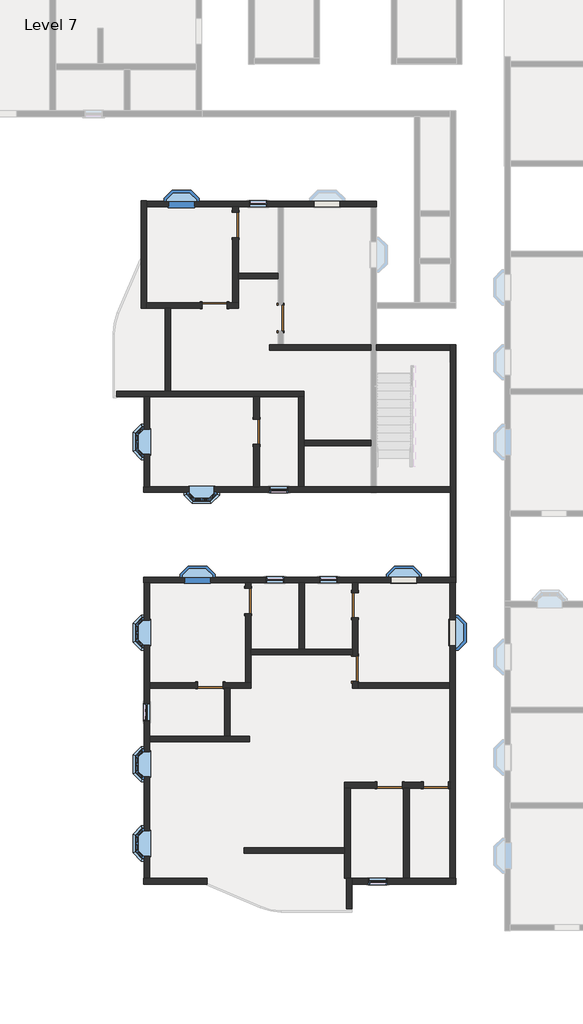
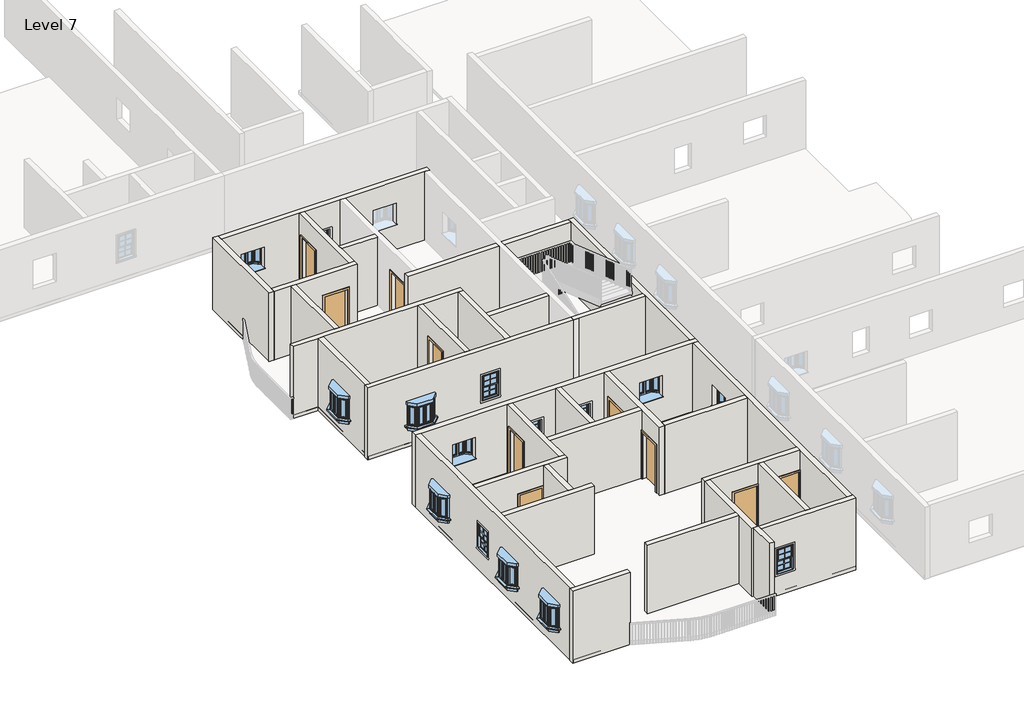
# One storey, part 1 of 14: 32 walls, 15 windows, 10 doors.
"""IFC4 building model written with IfcOpenShell, lengths in millimetres."""

from ifc_helpers import new_model, si_unit, frame, origin, place, context, project, spatial, polyline, outline, extrude, faceted_brep, transform, mapped, element, save
from components import door_54dd4da4, door_719f80de, window_910x910mm_67ef725a, window_8debb0fa

model = new_model("IFC4")

# Units and contexts
model_context = context("Model", 3, world=origin())
ifc_project = project(units=[si_unit("LENGTHUNIT", "METRE", prefix="MILLI")], contexts=[model_context])

# Site, building, storey
site = spatial("IfcSite", under=ifc_project)
building = spatial("IfcBuilding", under=site)
storey = spatial("IfcBuildingStorey", under=building, Name="Level 7", Elevation=18288.0)

# Doors
placement = place(None, origin())
door_shape = door_54dd4da4(model_context)
element("IfcDoor", 1, ObjectType="Single-Flush : 36\" x 84\"", at=placement, inside=storey, context=model_context, shape_type="MappedRepresentation", body=[
    mapped(door_shape, transform((-4626.037215, -17283.4916506, 18288.0), x_axis=(0.0, -1.0, 0.0), y_axis=(1.0, 0.0, 0.0), z_axis=(0.0, 0.0, 1.0))),
])
element("IfcDoor", 2, ObjectType="Single-Flush : 36\" x 84\"", at=placement, inside=storey, context=model_context, shape_type="MappedRepresentation", body=[
    mapped(door_shape, transform((-4626.037215, -14978.4416506, 18288.0), x_axis=(0.0, 1.0, 0.0), y_axis=(-1.0, 0.0, 0.0), z_axis=(0.0, 0.0, 1.0))),
])
element("IfcDoor", 3, ObjectType="Single-Flush : 36\" x 84\"", at=placement, inside=storey, context=model_context, shape_type="MappedRepresentation", body=[
    mapped(door_shape, transform((-9731.437215, -4100.8916506, 18288.0), x_axis=(1.0, 0.0, 0.0), y_axis=(0.0, 1.0, 0.0), z_axis=(0.0, 0.0, 1.0))),
])
element("IfcDoor", 4, ObjectType="Single-Flush : 36\" x 84\"", at=placement, inside=storey, context=model_context, shape_type="MappedRepresentation", body=[
    mapped(door_shape, transform((-7331.137215, -4558.0916506, 18288.0), x_axis=(0.0, -1.0, 0.0), y_axis=(1.0, 0.0, 0.0), z_axis=(0.0, 0.0, 1.0))),
])
door_2_shape = door_719f80de(model_context)
element("IfcDoor", 5, ObjectType="Single-Flush : 36\" x 84\"", at=placement, inside=storey, context=model_context, shape_type="MappedRepresentation", body=[
    mapped(door_2_shape, transform((-9883.837215, -17891.2072331, 18288.0), x_axis=(1.0, 0.0, 0.0), y_axis=(0.0, 1.0, 0.0), z_axis=(0.0, 0.0, 1.0))),
])
element("IfcDoor", 6, ObjectType="Single-Flush : 36\" x 84\"", at=placement, inside=storey, context=model_context, shape_type="MappedRepresentation", body=[
    mapped(door_2_shape, transform((-8512.237215, -14826.0416506, 18288.0), x_axis=(0.0, 1.0, 0.0), y_axis=(-1.0, 0.0, 0.0), z_axis=(0.0, 0.0, 1.0))),
])
element("IfcDoor", 7, ObjectType="Single-Flush : 36\" x 84\"", at=placement, inside=storey, context=model_context, shape_type="MappedRepresentation", body=[
    mapped(door_2_shape, transform((-8207.437215, -8691.9416506, 18288.0), x_axis=(0.0, 1.0, 0.0), y_axis=(-1.0, 0.0, 0.0), z_axis=(0.0, 0.0, 1.0))),
])
element("IfcDoor", 8, ObjectType="Single-Flush : 36\" x 84\"", at=placement, inside=storey, context=model_context, shape_type="MappedRepresentation", body=[
    mapped(door_2_shape, transform((-8969.437215, -1186.2416506, 18288.0), x_axis=(0.0, 1.0, 0.0), y_axis=(-1.0, 0.0, 0.0), z_axis=(0.0, 0.0, 1.0))),
])
element("IfcDoor", 9, ObjectType="Single-Flush : 36\" x 84\"", at=placement, inside=storey, context=model_context, shape_type="MappedRepresentation", body=[
    mapped(door_2_shape, transform((-3374.4891351, -21512.5916506, 18288.0), x_axis=(1.0, 0.0, 0.0), y_axis=(0.0, 1.0, 0.0), z_axis=(0.0, 0.0, 1.0))),
])
element("IfcDoor", 10, ObjectType="Single-Flush : 36\" x 84\"", at=placement, inside=storey, context=model_context, shape_type="MappedRepresentation", body=[
    mapped(door_2_shape, transform((-1698.0891351, -21512.5916506, 18288.0), x_axis=(1.0, 0.0, 0.0), y_axis=(0.0, 1.0, 0.0), z_axis=(0.0, 0.0, 1.0))),
])

# Walls
element("IfcWall", 11, ObjectType="4.5\" p", at=placement, inside=storey, context=model_context, shape_type="Brep", body=[
    faceted_brep([(-9426.637215, -17992.8072331, 20421.6), (-9426.637215, -17992.8072331, 18288.0), (-9375.837215, -17992.8072331, 18288.0), (-9172.637215, -17992.8072331, 18288.0), (-8410.637215, -17992.8072331, 18288.0), (-8410.637215, -17992.8072331, 21336.0), (-9172.637215, -17992.8072331, 21336.0), (-9375.837215, -17992.8072331, 21336.0), (-12087.287215, -17992.8072331, 21336.0), (-12087.287215, -17992.8072331, 18288.0), (-10341.037215, -17992.8072331, 18288.0), (-10341.037215, -17992.8072331, 20421.6), (-8410.637215, -17789.6072331, 18288.0), (-8613.837215, -17789.6072331, 18288.0), (-9426.637215, -17789.6072331, 18288.0), (-9426.637215, -17789.6072331, 20421.6), (-10341.037215, -17789.6072331, 20421.6), (-10341.037215, -17789.6072331, 18288.0), (-12087.287215, -17789.6072331, 18288.0), (-12087.287215, -17789.6072331, 21336.0), (-8613.837215, -17789.6072331, 21336.0), (-8410.637215, -17789.6072331, 21336.0)], [[[0, 1, 2, 3, 4, 5, 6, 7, 8, 9, 10, 11]], [[12, 13, 14, 15, 16, 17, 18, 19, 20, 21]], [[10, 9, 18, 17]], [[4, 3, 2, 1, 14, 13, 12]], [[8, 7, 6, 5, 21, 20, 19]], [[9, 8, 19, 18]], [[5, 4, 12, 21]], [[15, 14, 1, 0]], [[16, 15, 0, 11]], [[17, 16, 11, 10]]]),
])
element("IfcWall", 12, ObjectType="4.5\" p", at=placement, inside=storey, context=model_context, shape_type="Brep", body=[
    faceted_brep([(-8410.637215, -14368.8416506, 20421.6), (-8410.637215, -14368.8416506, 18288.0), (-8410.637215, -14165.6416506, 18288.0), (-8410.637215, -14165.6416506, 21336.0), (-8410.637215, -16572.2916506, 21336.0), (-8410.637215, -16775.4916506, 21336.0), (-8410.637215, -17789.6072331, 21336.0), (-8410.637215, -17789.6072331, 18288.0), (-8410.637215, -16775.4916506, 18288.0), (-8410.637215, -16572.2916506, 18288.0), (-8410.637215, -15283.2416506, 18288.0), (-8410.637215, -15283.2416506, 20421.6), (-8613.837215, -14165.6416506, 18288.0), (-8613.837215, -14368.8416506, 18288.0), (-8613.837215, -14368.8416506, 20421.6), (-8613.837215, -15283.2416506, 20421.6), (-8613.837215, -15283.2416506, 18288.0), (-8613.837215, -17789.6072331, 18288.0), (-8613.837215, -17789.6072331, 21336.0), (-8613.837215, -14165.6416506, 21336.0)], [[[0, 1, 2, 3, 4, 5, 6, 7, 8, 9, 10, 11]], [[12, 13, 14, 15, 16, 17, 18, 19]], [[2, 1, 13, 12]], [[10, 9, 8, 7, 17, 16]], [[6, 5, 4, 3, 19, 18]], [[7, 6, 18, 17]], [[3, 2, 12, 19]], [[14, 13, 1, 0]], [[15, 14, 0, 11]], [[16, 15, 11, 10]]]),
])
element("IfcWall", 13, ObjectType="4.5\" p", at=placement, inside=storey, context=model_context, shape_type="Brep", body=[
    faceted_brep([(-8410.637215, -16775.4916506, 18288.0), (-4727.637215, -16775.4916506, 18288.0), (-4727.637215, -16775.4916506, 21336.0), (-8410.637215, -16775.4916506, 21336.0), (-8410.637215, -16572.2916506, 18288.0), (-8410.637215, -16572.2916506, 21336.0), (-6670.737215, -16572.2916506, 21336.0), (-6467.537215, -16572.2916506, 21336.0), (-4727.637215, -16572.2916506, 21336.0), (-4727.637215, -16572.2916506, 18288.0), (-6467.537215, -16572.2916506, 18288.0), (-6670.737215, -16572.2916506, 18288.0)], [[[0, 1, 2, 3]], [[4, 5, 6, 7, 8, 9, 10, 11]], [[1, 0, 4, 11, 10, 9]], [[3, 2, 8, 7, 6, 5]], [[0, 3, 5, 4]], [[2, 1, 9, 8]]]),
])
element("IfcWall", 14, ObjectType="4.5\" p", at=placement, inside=storey, context=model_context, shape_type="SweptSolid", body=[
    extrude(outline(polyline([(-6670.737215, -16572.2916506), (-6670.737215, -14165.6416506), (-6467.537215, -14165.6416506), (-6467.537215, -16572.2916506), (-6670.737215, -16572.2916506)])), frame((0.0, 0.0, 18288.0), z_axis=(0.0, 0.0, 1.0), x_axis=(1.0, 0.0, 0.0)), (0.0, 0.0, 1.0), 3048.0),
])
element("IfcWall", 15, ObjectType="4.5\" p", at=placement, inside=storey, context=model_context, shape_type="Brep", body=[
    faceted_brep([(-4727.637215, -14165.6416506, 18288.0), (-4727.637215, -14521.2416506, 18288.0), (-4727.637215, -14521.2416506, 20421.6), (-4727.637215, -15435.6416506, 20421.6), (-4727.637215, -15435.6416506, 18288.0), (-4727.637215, -16572.2916506, 18288.0), (-4727.637215, -16775.4916506, 18288.0), (-4727.637215, -16826.2916506, 18288.0), (-4727.637215, -16826.2916506, 20421.6), (-4727.637215, -17740.6916506, 20421.6), (-4727.637215, -17740.6916506, 18288.0), (-4727.637215, -17994.6916506, 18288.0), (-4727.637215, -17994.6916506, 21336.0), (-4727.637215, -16775.4916506, 21336.0), (-4727.637215, -16572.2916506, 21336.0), (-4727.637215, -14165.6416506, 21336.0), (-4524.437215, -14521.2416506, 20421.6), (-4524.437215, -14521.2416506, 18288.0), (-4524.437215, -14165.6416506, 18288.0), (-4524.437215, -14165.6416506, 21336.0), (-4524.437215, -17791.4916506, 21336.0), (-4524.437215, -17994.6916506, 21336.0), (-4524.437215, -17994.6916506, 18288.0), (-4524.437215, -17791.4916506, 18288.0), (-4524.437215, -17740.6916506, 18288.0), (-4524.437215, -17740.6916506, 20421.6), (-4524.437215, -16826.2916506, 20421.6), (-4524.437215, -16826.2916506, 18288.0), (-4524.437215, -15435.6416506, 18288.0), (-4524.437215, -15435.6416506, 20421.6)], [[[0, 1, 2, 3, 4, 5, 6, 7, 8, 9, 10, 11, 12, 13, 14, 15]], [[16, 17, 18, 19, 20, 21, 22, 23, 24, 25, 26, 27, 28, 29]], [[11, 10, 24, 23, 22]], [[28, 27, 7, 6, 5, 4]], [[18, 17, 1, 0]], [[15, 14, 13, 12, 21, 20, 19]], [[0, 15, 19, 18]], [[12, 11, 22, 21]], [[25, 24, 10, 9]], [[26, 25, 9, 8]], [[27, 26, 8, 7]], [[2, 1, 17, 16]], [[3, 2, 16, 29]], [[4, 3, 29, 28]]]),
])
element("IfcWall", 16, ObjectType="4.5\" p", at=placement, inside=storey, context=model_context, shape_type="SweptSolid", body=[
    extrude(outline(polyline([(-4524.437215, -17791.4916506), (-1190.0891351, -17791.4916506), (-1190.0891351, -17994.6916506), (-4524.437215, -17994.6916506), (-4524.437215, -17791.4916506)])), frame((0.0, 0.0, 18288.0), z_axis=(0.0, 0.0, 1.0), x_axis=(1.0, 0.0, 0.0)), (0.0, 0.0, 1.0), 3048.0),
])
element("IfcWall", 17, ObjectType="4.5\" p", at=placement, inside=storey, context=model_context, shape_type="SweptSolid", body=[
    extrude(outline(polyline([(-9375.837215, -19734.5916506), (-9375.837215, -17992.8072331), (-9172.637215, -17992.8072331), (-9172.637215, -19734.5916506), (-9375.837215, -19734.5916506)])), frame((0.0, 0.0, 18288.0), z_axis=(0.0, 0.0, 1.0), x_axis=(1.0, 0.0, 0.0)), (0.0, 0.0, 1.0), 3048.0),
])
element("IfcWall", 18, ObjectType="4.5\" p", at=placement, inside=storey, context=model_context, shape_type="Brep", body=[
    faceted_brep([(-12087.287215, -19937.7916506, 18288.0), (-8455.087215, -19937.7916506, 18288.0), (-8455.087215, -19937.7916506, 21336.0), (-12087.287215, -19937.7916506, 21336.0), (-12087.287215, -19734.5916506, 18288.0), (-12087.287215, -19734.5916506, 21336.0), (-9375.837215, -19734.5916506, 21336.0), (-9172.637215, -19734.5916506, 21336.0), (-8455.087215, -19734.5916506, 21336.0), (-8455.087215, -19734.5916506, 18288.0), (-9172.637215, -19734.5916506, 18288.0), (-9375.837215, -19734.5916506, 18288.0)], [[[0, 1, 2, 3]], [[4, 5, 6, 7, 8, 9, 10, 11]], [[1, 0, 4, 11, 10, 9]], [[2, 1, 9, 8]], [[3, 2, 8, 7, 6, 5]], [[0, 3, 5, 4]]]),
])
element("IfcWall", 19, ObjectType="4.5\" p", at=placement, inside=storey, context=model_context, shape_type="Brep", body=[
    faceted_brep([(-13293.787215, -7421.9416506, 18288.0), (-12290.487215, -7421.9416506, 18288.0), (-12087.287215, -7421.9416506, 18288.0), (-8309.037215, -7421.9416506, 18288.0), (-8105.837215, -7421.9416506, 18288.0), (-6689.787215, -7421.9416506, 18288.0), (-6486.587215, -7421.9416506, 18288.0), (-6486.587215, -7421.9416506, 21336.0), (-6689.787215, -7421.9416506, 21336.0), (-8105.837215, -7421.9416506, 21336.0), (-8309.037215, -7421.9416506, 21336.0), (-12087.287215, -7421.9416506, 21336.0), (-12290.487215, -7421.9416506, 21336.0), (-13293.787215, -7421.9416506, 21336.0), (-13293.787215, -7218.7416506, 18288.0), (-13293.787215, -7218.7416506, 21336.0), (-11528.487215, -7218.7416506, 21336.0), (-11325.287215, -7218.7416506, 21336.0), (-6486.587215, -7218.7416506, 21336.0), (-6486.587215, -7218.7416506, 18288.0), (-11325.287215, -7218.7416506, 18288.0), (-11528.487215, -7218.7416506, 18288.0)], [[[0, 1, 2, 3, 4, 5, 6, 7, 8, 9, 10, 11, 12, 13]], [[14, 15, 16, 17, 18, 19, 20, 21]], [[6, 5, 4, 3, 2, 1, 0, 14, 21, 20, 19]], [[13, 12, 11, 10, 9, 8, 7, 18, 17, 16, 15]], [[0, 13, 15, 14]], [[7, 6, 19, 18]]]),
])
element("IfcWall", 20, ObjectType="4.5\" p", at=placement, inside=storey, context=model_context, shape_type="Brep", body=[
    faceted_brep([(-12201.587215, -4202.4916506, 18288.0), (-12201.587215, -3999.2916506, 18288.0), (-12201.587215, -525.8416506, 18288.0), (-12201.587215, -322.6416506, 18288.0), (-12201.587215, -309.9416506, 18288.0), (-12201.587215, -309.9416506, 21336.0), (-12201.587215, -322.6416506, 21336.0), (-12201.587215, -525.8416506, 21336.0), (-12201.587215, -3999.2916506, 21336.0), (-12201.587215, -4202.4916506, 21336.0), (-12404.787215, -4202.4916506, 18288.0), (-12404.787215, -4202.4916506, 21336.0), (-12404.787215, -309.9416506, 21336.0), (-12404.787215, -309.9416506, 18288.0)], [[[0, 1, 2, 3, 4, 5, 6, 7, 8, 9]], [[10, 11, 12, 13]], [[4, 3, 2, 1, 0, 10, 13]], [[5, 4, 13, 12]], [[9, 8, 7, 6, 5, 12, 11]], [[0, 9, 11, 10]]]),
])
element("IfcWall", 21, ObjectType="4.5\" p", at=placement, inside=storey, context=model_context, shape_type="Brep", body=[
    faceted_brep([(-9274.237215, -4202.4916506, 20421.6), (-9274.237215, -4202.4916506, 18288.0), (-8867.837215, -4202.4916506, 18288.0), (-8867.837215, -4202.4916506, 21336.0), (-11325.287215, -4202.4916506, 21336.0), (-11528.487215, -4202.4916506, 21336.0), (-12201.587215, -4202.4916506, 21336.0), (-12201.587215, -4202.4916506, 18288.0), (-11528.487215, -4202.4916506, 18288.0), (-11325.287215, -4202.4916506, 18288.0), (-10188.637215, -4202.4916506, 18288.0), (-10188.637215, -4202.4916506, 20421.6), (-8867.837215, -3999.2916506, 18288.0), (-9071.037215, -3999.2916506, 18288.0), (-9274.237215, -3999.2916506, 18288.0), (-9274.237215, -3999.2916506, 20421.6), (-10188.637215, -3999.2916506, 20421.6), (-10188.637215, -3999.2916506, 18288.0), (-12201.587215, -3999.2916506, 18288.0), (-12201.587215, -3999.2916506, 21336.0), (-9071.037215, -3999.2916506, 21336.0), (-8867.837215, -3999.2916506, 21336.0)], [[[0, 1, 2, 3, 4, 5, 6, 7, 8, 9, 10, 11]], [[12, 13, 14, 15, 16, 17, 18, 19, 20, 21]], [[2, 1, 14, 13, 12]], [[10, 9, 8, 7, 18, 17]], [[6, 5, 4, 3, 21, 20, 19]], [[7, 6, 19, 18]], [[3, 2, 12, 21]], [[15, 14, 1, 0]], [[16, 15, 0, 11]], [[17, 16, 11, 10]]]),
])
element("IfcWall", 22, ObjectType="4.5\" p", at=placement, inside=storey, context=model_context, shape_type="Brep", body=[
    faceted_brep([(-8867.837215, -729.0416506, 20421.6), (-8867.837215, -729.0416506, 18288.0), (-8867.837215, -525.8416506, 18288.0), (-8867.837215, -525.8416506, 21336.0), (-8867.837215, -2932.4916506, 21336.0), (-8867.837215, -3135.6916506, 21336.0), (-8867.837215, -3999.2916506, 21336.0), (-8867.837215, -3999.2916506, 18288.0), (-8867.837215, -3135.6916506, 18288.0), (-8867.837215, -2932.4916506, 18288.0), (-8867.837215, -1643.4416506, 18288.0), (-8867.837215, -1643.4416506, 20421.6), (-9071.037215, -525.8416506, 18288.0), (-9071.037215, -729.0416506, 18288.0), (-9071.037215, -729.0416506, 20421.6), (-9071.037215, -1643.4416506, 20421.6), (-9071.037215, -1643.4416506, 18288.0), (-9071.037215, -3999.2916506, 18288.0), (-9071.037215, -3999.2916506, 21336.0), (-9071.037215, -525.8416506, 21336.0)], [[[0, 1, 2, 3, 4, 5, 6, 7, 8, 9, 10, 11]], [[12, 13, 14, 15, 16, 17, 18, 19]], [[2, 1, 13, 12]], [[10, 9, 8, 7, 17, 16]], [[6, 5, 4, 3, 19, 18]], [[7, 6, 18, 17]], [[3, 2, 12, 19]], [[14, 13, 1, 0]], [[15, 14, 0, 11]], [[16, 15, 11, 10]]]),
])
element("IfcWall", 23, ObjectType="4.5\" p", at=placement, inside=storey, context=model_context, shape_type="SweptSolid", body=[
    extrude(outline(polyline([(-7432.737215, -3135.6916506), (-8867.837215, -3135.6916506), (-8867.837215, -2932.4916506), (-7432.737215, -2932.4916506), (-7432.737215, -3135.6916506)])), frame((0.0, 0.0, 18288.0), z_axis=(0.0, 0.0, 1.0), x_axis=(1.0, 0.0, 0.0)), (0.0, 0.0, 1.0), 3048.0),
])
element("IfcWall", 24, ObjectType="4.5\" p", at=placement, inside=storey, context=model_context, shape_type="Brep", body=[
    faceted_brep([(-7731.187215, -5726.4916506, 21336.0), (-7731.187215, -5726.4916506, 18288.0), (-4060.887215, -5726.4916506, 18288.0), (-4060.887215, -5726.4916506, 21336.0), (-7731.187215, -5523.2916506, 18288.0), (-7731.187215, -5523.2916506, 21336.0), (-7432.737215, -5523.2916506, 21336.0), (-7229.537215, -5523.2916506, 21336.0), (-4060.887215, -5523.2916506, 21336.0), (-4060.887215, -5523.2916506, 18288.0), (-7229.537215, -5523.2916506, 18288.0), (-7432.737215, -5523.2916506, 18288.0)], [[[0, 1, 2, 3]], [[4, 5, 6, 7, 8, 9, 10, 11]], [[1, 4, 11, 10, 9, 2]], [[5, 0, 3, 8, 7, 6]], [[1, 0, 5, 4]], [[3, 2, 9, 8]]]),
    faceted_brep([(-1177.3891351, -5726.4916506, 18288.0), (-1177.3891351, -5726.4916506, 21336.0), (-3857.687215, -5726.4916506, 21336.0), (-3857.687215, -5726.4916506, 18288.0), (-1177.3891351, -5523.2916506, 21336.0), (-1177.3891351, -5523.2916506, 18288.0), (-3857.687215, -5523.2916506, 18288.0), (-3857.687215, -5523.2916506, 21336.0)], [[[0, 1, 2, 3]], [[4, 5, 6, 7]], [[5, 0, 3, 6]], [[1, 4, 7, 2]], [[1, 0, 5, 4]], [[3, 2, 7, 6]]]),
])
element("IfcWall", 25, ObjectType="4.5\" p", at=placement, inside=storey, context=model_context, shape_type="SweptSolid", body=[
    extrude(outline(polyline([(-11528.487215, -7218.7416506), (-11528.487215, -4202.4916506), (-11325.287215, -4202.4916506), (-11325.287215, -7218.7416506), (-11528.487215, -7218.7416506)])), frame((0.0, 0.0, 18288.0), z_axis=(0.0, 0.0, 1.0), x_axis=(1.0, 0.0, 0.0)), (0.0, 0.0, 1.0), 3048.0),
])
element("IfcWall", 26, ObjectType="4.5\" p", at=placement, inside=storey, context=model_context, shape_type="SweptSolid", body=[
    extrude(outline(polyline([(-7421.9416506, 18288.0), (-8234.7416506, 18288.0), (-8234.7416506, 20421.6), (-9149.1416506, 20421.6), (-9149.1416506, 18288.0), (-10685.8416506, 18288.0), (-10685.8416506, 21336.0), (-7421.9416506, 21336.0), (-7421.9416506, 18288.0)])), frame((-8309.037215, 0.0, 0.0), z_axis=(1.0, 0.0, 0.0), x_axis=(0.0, 1.0, 0.0)), (0.0, 0.0, 1.0), 203.2),
])
element("IfcWall", 27, ObjectType="4.5\" p", at=placement, inside=storey, context=model_context, shape_type="Brep", body=[
    faceted_brep([(-6689.787215, -7421.9416506, 18288.0), (-6689.787215, -10685.8416506, 18288.0), (-6689.787215, -10685.8416506, 21336.0), (-6689.787215, -7421.9416506, 21336.0), (-6486.587215, -7421.9416506, 18288.0), (-6486.587215, -7421.9416506, 21336.0), (-6486.587215, -8990.3916506, 21336.0), (-6486.587215, -9193.5916506, 21336.0), (-6486.587215, -10685.8416506, 21336.0), (-6486.587215, -10685.8416506, 18288.0), (-6486.587215, -9193.5916506, 18288.0), (-6486.587215, -8990.3916506, 18288.0)], [[[0, 1, 2, 3]], [[4, 5, 6, 7, 8, 9, 10, 11]], [[1, 0, 4, 11, 10, 9]], [[3, 2, 8, 7, 6, 5]], [[0, 3, 5, 4]], [[2, 1, 9, 8]]]),
])
element("IfcWall", 28, ObjectType="4.5\" p", at=placement, inside=storey, context=model_context, shape_type="SweptSolid", body=[
    extrude(outline(polyline([(-4060.887215, -9193.5916506), (-6486.587215, -9193.5916506), (-6486.587215, -8990.3916506), (-4060.887215, -8990.3916506), (-4060.887215, -9193.5916506)])), frame((0.0, 0.0, 18288.0), z_axis=(0.0, 0.0, 1.0), x_axis=(1.0, 0.0, 0.0)), (0.0, 0.0, 1.0), 3048.0),
])
element("IfcWall", 29, ObjectType="9\"", at=placement, inside=storey, context=model_context, shape_type="Brep", body=[
    faceted_brep([(-1190.0891351, -21410.9916506, 18288.0), (-1240.8891351, -21410.9916506, 18288.0), (-1240.8891351, -21410.9916506, 20421.6), (-2155.2891351, -21410.9916506, 20421.6), (-2155.2891351, -21410.9916506, 18288.0), (-2917.2891351, -21410.9916506, 18288.0), (-2917.2891351, -21410.9916506, 20421.6), (-3831.6891351, -21410.9916506, 20421.6), (-3831.6891351, -21410.9916506, 18288.0), (-5006.4391351, -21410.9916506, 18288.0), (-5006.4391351, -21410.9916506, 21336.0), (-1190.0891351, -21410.9916506, 21336.0), (-1240.8891351, -21614.1916506, 20421.6), (-1240.8891351, -21614.1916506, 18288.0), (-1190.0891351, -21614.1916506, 18288.0), (-1190.0891351, -21614.1916506, 21336.0), (-2663.2891351, -21614.1916506, 21336.0), (-2866.4891351, -21614.1916506, 21336.0), (-4803.2391351, -21614.1916506, 21336.0), (-5006.4391351, -21614.1916506, 21336.0), (-5006.4391351, -21614.1916506, 18288.0), (-4803.2391351, -21614.1916506, 18288.0), (-3831.6891351, -21614.1916506, 18288.0), (-3831.6891351, -21614.1916506, 20421.6), (-2917.2891351, -21614.1916506, 20421.6), (-2917.2891351, -21614.1916506, 18288.0), (-2866.4891351, -21614.1916506, 18288.0), (-2663.2891351, -21614.1916506, 18288.0), (-2155.2891351, -21614.1916506, 18288.0), (-2155.2891351, -21614.1916506, 20421.6)], [[[0, 1, 2, 3, 4, 5, 6, 7, 8, 9, 10, 11]], [[12, 13, 14, 15, 16, 17, 18, 19, 20, 21, 22, 23, 24, 25, 26, 27, 28, 29]], [[22, 21, 20, 9, 8]], [[14, 13, 1, 0]], [[28, 27, 26, 25, 5, 4]], [[11, 10, 19, 18, 17, 16, 15]], [[0, 11, 15, 14]], [[10, 9, 20, 19]], [[6, 5, 25, 24]], [[7, 6, 24, 23]], [[8, 7, 23, 22]], [[2, 1, 13, 12]], [[3, 2, 12, 29]], [[4, 3, 29, 28]]]),
])
element("IfcWall", 30, ObjectType="9\"", at=placement, inside=storey, context=model_context, shape_type="Brep", body=[
    faceted_brep([(-5006.4391351, -21614.1916506, 18288.0), (-5006.4391351, -23779.5416506, 18288.0), (-5006.4391351, -23982.7416506, 18288.0), (-5006.4391351, -24897.1416506, 18288.0), (-5006.4391351, -24897.1416506, 21336.0), (-5006.4391351, -23982.7416506, 21336.0), (-5006.4391351, -23779.5416506, 21336.0), (-5006.4391351, -21614.1916506, 21336.0), (-4803.2391351, -21614.1916506, 18288.0), (-4803.2391351, -21614.1916506, 21336.0), (-4803.2391351, -24897.1416506, 21336.0), (-4803.2391351, -24897.1416506, 18288.0), (-4949.2891351, -24897.1416506, 18288.0), (-4949.2891351, -24897.1416506, 21336.0)], [[[0, 1, 2, 3, 4, 5, 6, 7]], [[8, 9, 10, 11]], [[3, 2, 1, 0, 8, 11, 12]], [[7, 6, 5, 4, 13, 10, 9]], [[0, 7, 9, 8]], [[4, 3, 12, 11, 10, 13]]]),
])
element("IfcWall", 31, ObjectType="9\"", at=placement, inside=storey, context=model_context, shape_type="SweptSolid", body=[
    extrude(outline(polyline([(-2866.4891351, -24897.1416506), (-2866.4891351, -21614.1916506), (-2663.2891351, -21614.1916506), (-2663.2891351, -24897.1416506), (-2866.4891351, -24897.1416506)])), frame((0.0, 0.0, 18288.0), z_axis=(0.0, 0.0, 1.0), x_axis=(1.0, 0.0, 0.0)), (0.0, 0.0, 1.0), 3048.0),
])
element("IfcWall", 32, ObjectType="9\"", at=placement, inside=storey, context=model_context, shape_type="SweptSolid", body=[
    extrude(outline(polyline([(-5006.4391351, -23982.7416506), (-8664.637215, -23982.7416506), (-8664.637215, -23779.5416506), (-5006.4391351, -23779.5416506), (-5006.4391351, -23982.7416506)])), frame((0.0, 0.0, 18288.0), z_axis=(0.0, 0.0, 1.0), x_axis=(1.0, 0.0, 0.0)), (0.0, 0.0, 1.0), 3048.0),
])
element("IfcWall", 33, ObjectType="9\" w", at=placement, inside=storey, context=model_context, shape_type="Brep", body=[
    faceted_brep([(-12303.187215, -14165.6416506, 18288.0), (-12290.487215, -14165.6416506, 18288.0), (-12087.287215, -14165.6416506, 18288.0), (-8613.837215, -14165.6416506, 18288.0), (-8410.637215, -14165.6416506, 18288.0), (-6670.737215, -14165.6416506, 18288.0), (-6467.537215, -14165.6416506, 18288.0), (-4727.637215, -14165.6416506, 18288.0), (-4524.437215, -14165.6416506, 18288.0), (-1190.0891351, -14165.6416506, 18288.0), (-986.8891351, -14165.6416506, 18288.0), (-961.4891351, -14165.6416506, 18288.0), (-961.4891351, -14165.6416506, 21336.0), (-986.8891351, -14165.6416506, 21336.0), (-1190.0891351, -14165.6416506, 21336.0), (-4524.437215, -14165.6416506, 21336.0), (-4727.637215, -14165.6416506, 21336.0), (-6467.537215, -14165.6416506, 21336.0), (-6670.737215, -14165.6416506, 21336.0), (-8410.637215, -14165.6416506, 21336.0), (-8613.837215, -14165.6416506, 21336.0), (-12087.287215, -14165.6416506, 21336.0), (-12290.487215, -14165.6416506, 21336.0), (-12303.187215, -14165.6416506, 21336.0), (-10805.562215, -14165.6416506, 20398.0), (-9895.562215, -14165.6416506, 20398.0), (-9895.562215, -14165.6416506, 19488.0), (-10805.562215, -14165.6416506, 19488.0), (-3312.2631751, -14165.6416506, 20398.0), (-2402.2631751, -14165.6416506, 20398.0), (-2402.2631751, -14165.6416506, 19488.0), (-3312.2631751, -14165.6416506, 19488.0), (-7870.887215, -14165.6416506, 20269.2), (-7210.487215, -14165.6416506, 20269.2), (-7210.487215, -14165.6416506, 19202.4), (-7870.887215, -14165.6416506, 19202.4), (-5927.787215, -14165.6416506, 20269.2), (-5267.387215, -14165.6416506, 20269.2), (-5267.387215, -14165.6416506, 19202.4), (-5927.787215, -14165.6416506, 19202.4), (-12303.187215, -13962.4416506, 18288.0), (-12303.187215, -13962.4416506, 21336.0), (-1177.3891351, -13962.4416506, 21336.0), (-974.1891351, -13962.4416506, 21336.0), (-961.4891351, -13962.4416506, 21336.0), (-961.4891351, -13962.4416506, 18288.0), (-974.1891351, -13962.4416506, 18288.0), (-1177.3891351, -13962.4416506, 18288.0), (-10805.562215, -13962.4416506, 20398.0), (-10805.562215, -13962.4416506, 19488.0), (-9895.562215, -13962.4416506, 19488.0), (-9895.562215, -13962.4416506, 20398.0), (-3312.2631751, -13962.4416506, 20398.0), (-3312.2631751, -13962.4416506, 19488.0), (-2402.2631751, -13962.4416506, 19488.0), (-2402.2631751, -13962.4416506, 20398.0), (-7870.887215, -13962.4416506, 20269.2), (-7870.887215, -13962.4416506, 19202.4), (-7210.487215, -13962.4416506, 19202.4), (-7210.487215, -13962.4416506, 20269.2), (-5927.787215, -13962.4416506, 20269.2), (-5927.787215, -13962.4416506, 19202.4), (-5267.387215, -13962.4416506, 19202.4), (-5267.387215, -13962.4416506, 20269.2)], [[[0, 1, 2, 3, 4, 5, 6, 7, 8, 9, 10, 11, 12, 13, 14, 15, 16, 17, 18, 19, 20, 21, 22, 23], [24, 25, 26, 27], [28, 29, 30, 31], [32, 33, 34, 35], [36, 37, 38, 39]], [[40, 41, 42, 43, 44, 45, 46, 47], [48, 49, 50, 51], [52, 53, 54, 55], [56, 57, 58, 59], [60, 61, 62, 63]], [[11, 10, 9, 8, 7, 6, 5, 4, 3, 2, 1, 0, 40, 47, 46, 45]], [[12, 11, 45, 44]], [[23, 22, 21, 20, 19, 18, 17, 16, 15, 14, 13, 12, 44, 43, 42, 41]], [[0, 23, 41, 40]], [[49, 48, 24, 27]], [[50, 49, 27, 26]], [[51, 50, 26, 25]], [[48, 51, 25, 24]], [[53, 52, 28, 31]], [[54, 53, 31, 30]], [[55, 54, 30, 29]], [[52, 55, 29, 28]], [[57, 56, 32, 35]], [[58, 57, 35, 34]], [[59, 58, 34, 33]], [[56, 59, 33, 32]], [[61, 60, 36, 39]], [[62, 61, 39, 38]], [[63, 62, 38, 37]], [[60, 63, 37, 36]]]),
])
element("IfcWall", 34, ObjectType="9\" w", at=placement, inside=storey, context=model_context, shape_type="Brep", body=[
    faceted_brep([(-10004.0323936, -24897.1416506, 18288.0), (-12087.287215, -24897.1416506, 18288.0), (-12290.487215, -24897.1416506, 18288.0), (-12303.187215, -24897.1416506, 18288.0), (-12303.187215, -24897.1416506, 21336.0), (-12290.487215, -24897.1416506, 21336.0), (-12087.287215, -24897.1416506, 21336.0), (-10004.0323936, -24897.1416506, 21336.0), (-10004.0323936, -25100.3416506, 18288.0), (-10004.0323936, -25100.3416506, 21336.0), (-12303.187215, -25100.3416506, 21336.0), (-12303.187215, -25100.3416506, 18288.0)], [[[0, 1, 2, 3, 4, 5, 6, 7]], [[8, 9, 10, 11]], [[3, 2, 1, 0, 8, 11]], [[4, 3, 11, 10]], [[7, 6, 5, 4, 10, 9]], [[0, 7, 9, 8]]]),
])
element("IfcWall", 35, ObjectType="9\" w", at=placement, inside=storey, context=model_context, shape_type="Brep", body=[
    faceted_brep([(-4746.0891351, -25989.3416506, 18288.0), (-4746.0891351, -25100.3416506, 18288.0), (-4746.0891351, -24897.1416506, 18288.0), (-4746.0891351, -24897.1416506, 21336.0), (-4746.0891351, -25100.3416506, 21336.0), (-4746.0891351, -25989.3416506, 21336.0), (-4949.2891351, -25989.3416506, 18288.0), (-4949.2891351, -25989.3416506, 21336.0), (-4949.2891351, -24897.1416506, 21336.0), (-4949.2891351, -24897.1416506, 18288.0), (-4803.2391351, -24897.1416506, 18288.0), (-4803.2391351, -24897.1416506, 21336.0)], [[[0, 1, 2, 3, 4, 5]], [[6, 7, 8, 9]], [[2, 1, 0, 6, 9, 10]], [[5, 4, 3, 11, 8, 7]], [[0, 5, 7, 6]], [[3, 2, 10, 9, 8, 11]]]),
])
element("IfcWall", 36, ObjectType="9\" w", at=placement, inside=storey, context=model_context, shape_type="Brep", body=[
    faceted_brep([(-4746.0891351, -25100.3416506, 18288.0), (-961.4891351, -25100.3416506, 18288.0), (-961.4891351, -25100.3416506, 21336.0), (-4746.0891351, -25100.3416506, 21336.0), (-3476.0891351, -25100.3416506, 20269.2), (-3476.0891351, -25100.3416506, 19202.4), (-4136.4891351, -25100.3416506, 19202.4), (-4136.4891351, -25100.3416506, 20269.2), (-4746.0891351, -24897.1416506, 18288.0), (-4746.0891351, -24897.1416506, 21336.0), (-2866.4891351, -24897.1416506, 21336.0), (-2663.2891351, -24897.1416506, 21336.0), (-1190.0891351, -24897.1416506, 21336.0), (-986.8891351, -24897.1416506, 21336.0), (-961.4891351, -24897.1416506, 21336.0), (-961.4891351, -24897.1416506, 18288.0), (-986.8891351, -24897.1416506, 18288.0), (-1190.0891351, -24897.1416506, 18288.0), (-2663.2891351, -24897.1416506, 18288.0), (-2866.4891351, -24897.1416506, 18288.0), (-3476.0891351, -24897.1416506, 20269.2), (-4136.4891351, -24897.1416506, 20269.2), (-4136.4891351, -24897.1416506, 19202.4), (-3476.0891351, -24897.1416506, 19202.4)], [[[0, 1, 2, 3], [4, 5, 6, 7]], [[8, 9, 10, 11, 12, 13, 14, 15, 16, 17, 18, 19], [20, 21, 22, 23]], [[1, 0, 8, 19, 18, 17, 16, 15]], [[2, 1, 15, 14]], [[3, 2, 14, 13, 12, 11, 10, 9]], [[0, 3, 9, 8]], [[5, 4, 20, 23]], [[6, 5, 23, 22]], [[7, 6, 22, 21]], [[4, 7, 21, 20]]]),
])
element("IfcWall", 37, ObjectType="9\" w", at=placement, inside=storey, context=model_context, shape_type="Brep", body=[
    faceted_brep([(-12290.487215, -14165.6416506, 18288.0), (-12290.487215, -24897.1416506, 18288.0), (-12290.487215, -24897.1416506, 21336.0), (-12290.487215, -14165.6416506, 21336.0), (-12290.487215, -16432.6244419, 20112.4), (-12290.487215, -16432.6244419, 19202.4), (-12290.487215, -15522.6244419, 19202.4), (-12290.487215, -15522.6244419, 20112.4), (-12290.487215, -21205.5916506, 20112.4), (-12290.487215, -21205.5916506, 19202.4), (-12290.487215, -20295.5916506, 19202.4), (-12290.487215, -20295.5916506, 20112.4), (-12290.487215, -24082.1416506, 20112.4), (-12290.487215, -24082.1416506, 19202.4), (-12290.487215, -23172.1416506, 19202.4), (-12290.487215, -23172.1416506, 20112.4), (-12290.487215, -19193.8994419, 20269.2), (-12290.487215, -19193.8994419, 19202.4), (-12290.487215, -18533.4994419, 19202.4), (-12290.487215, -18533.4994419, 20269.2), (-12087.287215, -14165.6416506, 18288.0), (-12087.287215, -14165.6416506, 21336.0), (-12087.287215, -17789.6072331, 21336.0), (-12087.287215, -17992.8072331, 21336.0), (-12087.287215, -19734.5916506, 21336.0), (-12087.287215, -19937.7916506, 21336.0), (-12087.287215, -24897.1416506, 21336.0), (-12087.287215, -24897.1416506, 18288.0), (-12087.287215, -19937.7916506, 18288.0), (-12087.287215, -19734.5916506, 18288.0), (-12087.287215, -17992.8072331, 18288.0), (-12087.287215, -17789.6072331, 18288.0), (-12087.287215, -16432.6244419, 20112.4), (-12087.287215, -15522.6244419, 20112.4), (-12087.287215, -15522.6244419, 19202.4), (-12087.287215, -16432.6244419, 19202.4), (-12087.287215, -21205.5916506, 20112.4), (-12087.287215, -20295.5916506, 20112.4), (-12087.287215, -20295.5916506, 19202.4), (-12087.287215, -21205.5916506, 19202.4), (-12087.287215, -24082.1416506, 20112.4), (-12087.287215, -23172.1416506, 20112.4), (-12087.287215, -23172.1416506, 19202.4), (-12087.287215, -24082.1416506, 19202.4), (-12087.287215, -19193.8994419, 20269.2), (-12087.287215, -18533.4994419, 20269.2), (-12087.287215, -18533.4994419, 19202.4), (-12087.287215, -19193.8994419, 19202.4)], [[[0, 1, 2, 3], [4, 5, 6, 7], [8, 9, 10, 11], [12, 13, 14, 15], [16, 17, 18, 19]], [[20, 21, 22, 23, 24, 25, 26, 27, 28, 29, 30, 31], [32, 33, 34, 35], [36, 37, 38, 39], [40, 41, 42, 43], [44, 45, 46, 47]], [[1, 0, 20, 31, 30, 29, 28, 27]], [[3, 2, 26, 25, 24, 23, 22, 21]], [[0, 3, 21, 20]], [[2, 1, 27, 26]], [[5, 4, 32, 35]], [[6, 5, 35, 34]], [[7, 6, 34, 33]], [[4, 7, 33, 32]], [[9, 8, 36, 39]], [[10, 9, 39, 38]], [[11, 10, 38, 37]], [[8, 11, 37, 36]], [[13, 12, 40, 43]], [[14, 13, 43, 42]], [[15, 14, 42, 41]], [[12, 15, 41, 40]], [[17, 16, 44, 47]], [[18, 17, 47, 46]], [[19, 18, 46, 45]], [[16, 19, 45, 44]]]),
])
element("IfcWall", 38, ObjectType="9\" w", at=placement, inside=storey, context=model_context, shape_type="Brep", body=[
    faceted_brep([(-1190.0891351, -14165.6416506, 18288.0), (-1190.0891351, -17791.4916506, 18288.0), (-1190.0891351, -17994.6916506, 18288.0), (-1190.0891351, -21410.9916506, 18288.0), (-1190.0891351, -21614.1916506, 18288.0), (-1190.0891351, -24897.1416506, 18288.0), (-1190.0891351, -24897.1416506, 21336.0), (-1190.0891351, -21614.1916506, 21336.0), (-1190.0891351, -21410.9916506, 21336.0), (-1190.0891351, -17994.6916506, 21336.0), (-1190.0891351, -17791.4916506, 21336.0), (-1190.0891351, -14165.6416506, 21336.0), (-1190.0891351, -15523.5666506, 20398.0), (-1190.0891351, -16433.5666506, 20398.0), (-1190.0891351, -16433.5666506, 19488.0), (-1190.0891351, -15523.5666506, 19488.0), (-986.8891351, -14165.6416506, 18288.0), (-986.8891351, -14165.6416506, 21336.0), (-986.8891351, -24897.1416506, 21336.0), (-986.8891351, -24897.1416506, 18288.0), (-986.8891351, -15523.5666506, 20398.0), (-986.8891351, -15523.5666506, 19488.0), (-986.8891351, -16433.5666506, 19488.0), (-986.8891351, -16433.5666506, 20398.0)], [[[0, 1, 2, 3, 4, 5, 6, 7, 8, 9, 10, 11], [12, 13, 14, 15]], [[16, 17, 18, 19], [20, 21, 22, 23]], [[5, 4, 3, 2, 1, 0, 16, 19]], [[11, 10, 9, 8, 7, 6, 18, 17]], [[0, 11, 17, 16]], [[6, 5, 19, 18]], [[21, 20, 12, 15]], [[22, 21, 15, 14]], [[23, 22, 14, 13]], [[20, 23, 13, 12]]]),
])
element("IfcWall", 39, ObjectType="9\" w", at=placement, inside=storey, context=model_context, shape_type="Brep", body=[
    faceted_brep([(-1177.3891351, -5523.2916506, 18288.0), (-1177.3891351, -5726.4916506, 18288.0), (-1177.3891351, -10685.8416506, 18288.0), (-1177.3891351, -10889.0416506, 18288.0), (-1177.3891351, -13962.4416506, 18288.0), (-1177.3891351, -13962.4416506, 21336.0), (-1177.3891351, -10889.0416506, 21336.0), (-1177.3891351, -10685.8416506, 21336.0), (-1177.3891351, -5726.4916506, 21336.0), (-1177.3891351, -5523.2916506, 21336.0), (-974.1891351, -5523.2916506, 18288.0), (-974.1891351, -5523.2916506, 21336.0), (-974.1891351, -13962.4416506, 21336.0), (-974.1891351, -13962.4416506, 18288.0)], [[[0, 1, 2, 3, 4, 5, 6, 7, 8, 9]], [[10, 11, 12, 13]], [[4, 3, 2, 1, 0, 10, 13]], [[9, 8, 7, 6, 5, 12, 11]], [[5, 4, 13, 12]], [[0, 9, 11, 10]]]),
])
element("IfcWall", 40, ObjectType="9\" w", at=placement, inside=storey, context=model_context, shape_type="Brep", body=[
    faceted_brep([(-1177.3891351, -10685.8416506, 18288.0), (-6486.587215, -10685.8416506, 18288.0), (-6689.787215, -10685.8416506, 18288.0), (-8105.837215, -10685.8416506, 18288.0), (-8309.037215, -10685.8416506, 18288.0), (-12087.287215, -10685.8416506, 18288.0), (-12290.487215, -10685.8416506, 18288.0), (-12303.187215, -10685.8416506, 18288.0), (-12303.187215, -10685.8416506, 21336.0), (-12290.487215, -10685.8416506, 21336.0), (-12087.287215, -10685.8416506, 21336.0), (-8309.037215, -10685.8416506, 21336.0), (-8105.837215, -10685.8416506, 21336.0), (-6689.787215, -10685.8416506, 21336.0), (-6486.587215, -10685.8416506, 21336.0), (-1177.3891351, -10685.8416506, 21336.0), (-9743.162215, -10685.8416506, 20112.4), (-10653.162215, -10685.8416506, 20112.4), (-10653.162215, -10685.8416506, 19202.4), (-9743.162215, -10685.8416506, 19202.4), (-7067.612215, -10685.8416506, 20269.2), (-7728.012215, -10685.8416506, 20269.2), (-7728.012215, -10685.8416506, 19202.4), (-7067.612215, -10685.8416506, 19202.4), (-1177.3891351, -10889.0416506, 18288.0), (-1177.3891351, -10889.0416506, 21336.0), (-12303.187215, -10889.0416506, 21336.0), (-12303.187215, -10889.0416506, 18288.0), (-9743.162215, -10889.0416506, 20112.4), (-9743.162215, -10889.0416506, 19202.4), (-10653.162215, -10889.0416506, 19202.4), (-10653.162215, -10889.0416506, 20112.4), (-7067.612215, -10889.0416506, 20269.2), (-7067.612215, -10889.0416506, 19202.4), (-7728.012215, -10889.0416506, 19202.4), (-7728.012215, -10889.0416506, 20269.2)], [[[0, 1, 2, 3, 4, 5, 6, 7, 8, 9, 10, 11, 12, 13, 14, 15], [16, 17, 18, 19], [20, 21, 22, 23]], [[24, 25, 26, 27], [28, 29, 30, 31], [32, 33, 34, 35]], [[7, 6, 5, 4, 3, 2, 1, 0, 24, 27]], [[8, 7, 27, 26]], [[15, 14, 13, 12, 11, 10, 9, 8, 26, 25]], [[0, 15, 25, 24]], [[29, 28, 16, 19]], [[30, 29, 19, 18]], [[31, 30, 18, 17]], [[28, 31, 17, 16]], [[33, 32, 20, 23]], [[34, 33, 23, 22]], [[35, 34, 22, 21]], [[32, 35, 21, 20]]]),
])
element("IfcWall", 41, ObjectType="9\" w", at=placement, inside=storey, context=model_context, shape_type="SweptSolid", body=[
    extrude(outline(polyline([(-10685.8416506, 18288.0), (-10685.8416506, 21336.0), (-7421.9416506, 21336.0), (-7421.9416506, 18288.0), (-10685.8416506, 18288.0)]), holes=[polyline([(-9508.8916506, 20112.4), (-9508.8916506, 19202.4), (-8598.8916506, 19202.4), (-8598.8916506, 20112.4), (-9508.8916506, 20112.4)])]), frame((-12290.487215, 0.0, 0.0), z_axis=(1.0, 0.0, 0.0), x_axis=(0.0, 1.0, 0.0)), (0.0, 0.0, 1.0), 203.2),
])
element("IfcWall", 42, ObjectType="9\" w", at=placement, inside=storey, context=model_context, shape_type="Brep", body=[
    faceted_brep([(-12201.587215, -525.8416506, 18288.0), (-9071.037215, -525.8416506, 18288.0), (-8867.837215, -525.8416506, 18288.0), (-7432.737215, -525.8416506, 18288.0), (-7229.537215, -525.8416506, 18288.0), (-4060.887215, -525.8416506, 18288.0), (-3857.687215, -525.8416506, 18288.0), (-3844.987215, -525.8416506, 18288.0), (-3844.987215, -525.8416506, 21336.0), (-3857.687215, -525.8416506, 21336.0), (-4060.887215, -525.8416506, 21336.0), (-7229.537215, -525.8416506, 21336.0), (-7432.737215, -525.8416506, 21336.0), (-8867.837215, -525.8416506, 21336.0), (-9071.037215, -525.8416506, 21336.0), (-12201.587215, -525.8416506, 21336.0), (-6100.212215, -525.8416506, 20398.0), (-5190.212215, -525.8416506, 20398.0), (-5190.212215, -525.8416506, 19488.0), (-6100.212215, -525.8416506, 19488.0), (-11386.587215, -525.8416506, 20398.0), (-10476.587215, -525.8416506, 20398.0), (-10476.587215, -525.8416506, 19488.0), (-11386.587215, -525.8416506, 19488.0), (-8480.487215, -525.8416506, 20269.2), (-7820.087215, -525.8416506, 20269.2), (-7820.087215, -525.8416506, 19202.4), (-8480.487215, -525.8416506, 19202.4), (-12201.587215, -322.6416506, 18288.0), (-12201.587215, -322.6416506, 21336.0), (-3844.987215, -322.6416506, 21336.0), (-3844.987215, -322.6416506, 18288.0), (-6100.212215, -322.6416506, 20398.0), (-6100.212215, -322.6416506, 19488.0), (-5190.212215, -322.6416506, 19488.0), (-5190.212215, -322.6416506, 20398.0), (-11386.587215, -322.6416506, 20398.0), (-11386.587215, -322.6416506, 19488.0), (-10476.587215, -322.6416506, 19488.0), (-10476.587215, -322.6416506, 20398.0), (-8480.487215, -322.6416506, 20269.2), (-8480.487215, -322.6416506, 19202.4), (-7820.087215, -322.6416506, 19202.4), (-7820.087215, -322.6416506, 20269.2)], [[[0, 1, 2, 3, 4, 5, 6, 7, 8, 9, 10, 11, 12, 13, 14, 15], [16, 17, 18, 19], [20, 21, 22, 23], [24, 25, 26, 27]], [[28, 29, 30, 31], [32, 33, 34, 35], [36, 37, 38, 39], [40, 41, 42, 43]], [[7, 6, 5, 4, 3, 2, 1, 0, 28, 31]], [[8, 7, 31, 30]], [[15, 14, 13, 12, 11, 10, 9, 8, 30, 29]], [[0, 15, 29, 28]], [[33, 32, 16, 19]], [[34, 33, 19, 18]], [[35, 34, 18, 17]], [[32, 35, 17, 16]], [[37, 36, 20, 23]], [[38, 37, 23, 22]], [[39, 38, 22, 21]], [[36, 39, 21, 20]], [[41, 40, 24, 27]], [[42, 41, 27, 26]], [[43, 42, 26, 25]], [[40, 43, 25, 24]]]),
])

# Windows
window_910x910mm_shape = window_910x910mm_67ef725a(model_context)
element("IfcWindow", 43, ObjectType="910x910mm", at=placement, inside=storey, context=model_context, shape_type="MappedRepresentation", body=[
    mapped(window_910x910mm_shape, transform((-10361.587215, -432.6982184, 18288.0), x_axis=(1.0, 0.0, 0.0), y_axis=(0.0, 1.0, 0.0), z_axis=(0.0, 0.0, 1.0))),
])
element("IfcWindow", 44, ObjectType="910x910mm", at=placement, inside=storey, context=model_context, shape_type="MappedRepresentation", body=[
    mapped(window_910x910mm_shape, transform((-12180.4306471, -8483.8916506, 18002.4), x_axis=(0.0, 1.0, 0.0), y_axis=(-1.0, 0.0, 0.0), z_axis=(0.0, 0.0, 1.0))),
])
element("IfcWindow", 45, ObjectType="910x910mm", at=placement, inside=storey, context=model_context, shape_type="MappedRepresentation", body=[
    mapped(window_910x910mm_shape, transform((-10768.162215, -10778.9850828, 18002.4), x_axis=(-1.0, 0.0, 0.0), y_axis=(0.0, -1.0, 0.0), z_axis=(0.0, 0.0, 1.0))),
])
element("IfcWindow", 46, ObjectType="910x910mm", at=placement, inside=storey, context=model_context, shape_type="MappedRepresentation", body=[
    mapped(window_910x910mm_shape, transform((-12180.4306471, -15407.6244419, 18002.4), x_axis=(0.0, 1.0, 0.0), y_axis=(-1.0, 0.0, 0.0), z_axis=(0.0, 0.0, 1.0))),
])
element("IfcWindow", 47, ObjectType="910x910mm", at=placement, inside=storey, context=model_context, shape_type="MappedRepresentation", body=[
    mapped(window_910x910mm_shape, transform((-9780.562215, -14072.4982184, 18288.0), x_axis=(1.0, 0.0, 0.0), y_axis=(0.0, 1.0, 0.0), z_axis=(0.0, 0.0, 1.0))),
])
element("IfcWindow", 48, ObjectType="910x910mm", at=placement, inside=storey, context=model_context, shape_type="MappedRepresentation", body=[
    mapped(window_910x910mm_shape, transform((-2287.2631751, -14072.4982184, 18288.0), x_axis=(1.0, 0.0, 0.0), y_axis=(0.0, 1.0, 0.0), z_axis=(0.0, 0.0, 1.0))),
])
element("IfcWindow", 49, ObjectType="910x910mm", at=placement, inside=storey, context=model_context, shape_type="MappedRepresentation", body=[
    mapped(window_910x910mm_shape, transform((-1096.945703, -16548.5666506, 18288.0), x_axis=(0.0, -1.0, 0.0), y_axis=(1.0, 0.0, 0.0), z_axis=(0.0, 0.0, 1.0))),
])
element("IfcWindow", 50, ObjectType="910x910mm", at=placement, inside=storey, context=model_context, shape_type="MappedRepresentation", body=[
    mapped(window_910x910mm_shape, transform((-12180.4306471, -20180.5916506, 18002.4), x_axis=(0.0, 1.0, 0.0), y_axis=(-1.0, 0.0, 0.0), z_axis=(0.0, 0.0, 1.0))),
])
element("IfcWindow", 51, ObjectType="910x910mm", at=placement, inside=storey, context=model_context, shape_type="MappedRepresentation", body=[
    mapped(window_910x910mm_shape, transform((-12180.4306471, -23057.1416506, 18002.4), x_axis=(0.0, 1.0, 0.0), y_axis=(-1.0, 0.0, 0.0), z_axis=(0.0, 0.0, 1.0))),
])
window_shape = window_8debb0fa(model_context)
element("IfcWindow", 52, ObjectType="Window-Double-Hung : 26\" x 42\"", at=placement, inside=storey, context=model_context, shape_type="MappedRepresentation", body=[
    mapped(window_shape, transform((-8150.287215, -424.2416506, 18288.0), x_axis=(1.0, 0.0, 0.0), y_axis=(0.0, 1.0, 0.0), z_axis=(0.0, 0.0, 1.0))),
])
element("IfcWindow", 53, ObjectType="Window-Double-Hung : 26\" x 42\"", at=placement, inside=storey, context=model_context, shape_type="MappedRepresentation", body=[
    mapped(window_shape, transform((-7397.812215, -10787.4416506, 18288.0), x_axis=(-1.0, 0.0, 0.0), y_axis=(0.0, -1.0, 0.0), z_axis=(0.0, 0.0, 1.0))),
])
element("IfcWindow", 54, ObjectType="Window-Double-Hung : 26\" x 42\"", at=placement, inside=storey, context=model_context, shape_type="MappedRepresentation", body=[
    mapped(window_shape, transform((-7540.687215, -14064.0416506, 18288.0), x_axis=(1.0, 0.0, 0.0), y_axis=(0.0, 1.0, 0.0), z_axis=(0.0, 0.0, 1.0))),
])
element("IfcWindow", 55, ObjectType="Window-Double-Hung : 26\" x 42\"", at=placement, inside=storey, context=model_context, shape_type="MappedRepresentation", body=[
    mapped(window_shape, transform((-5597.587215, -14064.0416506, 18288.0), x_axis=(1.0, 0.0, 0.0), y_axis=(0.0, 1.0, 0.0), z_axis=(0.0, 0.0, 1.0))),
])
element("IfcWindow", 56, ObjectType="Window-Double-Hung : 26\" x 42\"", at=placement, inside=storey, context=model_context, shape_type="MappedRepresentation", body=[
    mapped(window_shape, transform((-12188.887215, -18863.6994419, 18288.0), x_axis=(0.0, 1.0, 0.0), y_axis=(-1.0, 0.0, 0.0), z_axis=(0.0, 0.0, 1.0))),
])
element("IfcWindow", 57, ObjectType="Window-Double-Hung : 26\" x 42\"", at=placement, inside=storey, context=model_context, shape_type="MappedRepresentation", body=[
    mapped(window_shape, transform((-3806.2891351, -24998.7416506, 18288.0), x_axis=(-1.0, 0.0, 0.0), y_axis=(0.0, -1.0, 0.0), z_axis=(0.0, 0.0, 1.0))),
])

save(model, "model.ifc")

# Revit data of these elements
# Type "Single-Flush : 36\" x 84\""
#   Type Mark = "1"
#   Construction Type Id = "MDOOR"
#   Assembly Code = "C1020"
#   Analytic Construction = "Metal"
#   Thickness = 0' - 2"
#   Heat Transfer Coefficient (U) = 0.651978 BTU/(h·ft²·°F)
#   Height = 7' - 0"
#   Trim Projection Ext = 0' - 1"
#   Trim Projection Int = 0' - 1"
#   Trim Width = 0' - 3"
#   Width = 3' - 0"
#   Define Thermal Properties by = 1
#   Define Thermal Properties by = 1
#   Door Material = Door - Panel
#   Frame Material = Door - Frame
#   Visual Light Transmittance = 0
#   Solar Heat Gain Coefficient = 0
#   Function = (empty or 0)
#   Wall Closure = (empty or 0)
# Type "4.5\" p"
#   Assembly Code = "B2010"
#   Layers, outside or top first: 0' - 8" no material (function 1)
# Type "9\""
#   Assembly Code = "B2010"
#   Layers, outside or top first: 0' - 8" no material (function 1)
# Type "9\" w"
#   Assembly Code = "B2010"
#   Layers, outside or top first: 0' - 8" no material (function 1)
# Type "910x910mm"
#   Type Mark = "18"
#   Operation = "UserDefined"
#   Construction Type Id = "GSP4R"
#   Keynote = "L10"
#   Analytic Construction = "1/8 in Pilkington single glazing"
#   Wrap Layers (Ext) from Ext = 0' - 4.03543"
#   Wrap Layers (Int) from Ext = 0' - 6.98819"
#   Window Board Projection = 0' - 0.98425"
#   Window Board Extention = 0' - 0.98425"
#   Visual Light Transmittance = 0.9
#   Solar Heat Gain Coefficient = 0.78
#   Heat Transfer Coefficient (U) = 0.6496 BTU/(h·ft²·°F)
#   Glazing Thickness = 0' - 0.94488"
#   DONT CHANGE - Splay Width = 0' - 7.41997"
#   Rough Width = 2' - 11.82677"
#   Rough Height = 2' - 11.82677"
#   Roof Thickness = 0' - 4.92126"
#   Roof Overhang = 0' - 1.5748"
#   Plinth Thickness = 0' - 6.88976"
#   Height = 2' - 11.82677"
#   Width = 2' - 11.82677"
#   Frame Depth = 0' - 2.55906"
#   Default Head Height = 6' - 11.07087"
#   Cill Depth = 0' - 3.44488"
#   Cavity Closer Width = 0' - 1.9685"
#   Cavity Closer Offset from Ext = 0' - 4.03543"
#   Cavity Closer Depth = 0' - 3.34646"
#   Vis - Cavity Closers = yes
#   Define Thermal Properties by = 1
#   Material Trim = Window Frame
#   Material Glass = Glass
#   Material Frame = Window Frame
#   Manufacturer = ""
#   Wall Closure = (empty or 0)
# Type "Window-Double-Hung : 26\" x 42\""
#   Type Mark = "11"
#   Fire Rating = "0.5h"
#   Construction Type Id = "DG-DR"
#   Assembly Code = "B2020100"
#   Analytic Construction = "Double glazing - domestic"
#   Wall Thickness [instance default] = 0' - 6"
#   Window Inset [instance default] = 0' - 0"
#   Visual Light Transmittance = 0.81
#   Thermal Resistance (R) = 1.8146 (h·ft²·°F)/BTU
#   Solar Heat Gain Coefficient = 0.76
#   Muntin Width = 1' - 8"
#   Muntin Height = 1' - 5 1/8"
#   Interior Wall Closure [instance default] = 0' - 1 1/2"
#   Rough Width = 2' - 2 1/2"
#   Rough Height = 3' - 6 1/2"
#   Frame Extension [instance default] = 0' - 1 1/4"
#   Exterior Wall Closure [instance default] = 0' - 0 1/2"
#   Extension Jamb [instance default] = 0' - 1 1/2"
#   Heat Transfer Coefficient (U) = 0.5511 BTU/(h·ft²·°F)
#   Height = 3' - 6"
#   Width = 2' - 2"
#   Define Thermal Properties by = 1
#   Top Muntin Visibility = yes
#   Indicator Visibility [instance default] = yes
#   Extension Jamb Visibility [instance default] = yes
#   Interior Trim Visibility [instance default] = yes
#   Exterior Trim Visibility [instance default] = yes
#   Define Thermal Properties by = 1
#   Bottom Muntin Visibility = yes
#   Muntin Pattern = Muntin Pattern_2x2 : Muntin Pattern_2x2
#   Interior Trim Material = Wood - Stained
#   Interior Trim = Trim-Window-Interior-Flat : Picture Frame
#   Exterior Trim Material = Clad - White
#   Exterior Trim = Trim-Window-Exterior-Flat : with Sill
#   Glass Panel Material = Glass
#   Exterior Frame Material = Clad - White
#   Interior Frame Material = Wood - Stained
#   Wall Closure = (empty or 0)
# Elements 1, 2, 3, 4, 5, 6, 7, 8, 9, 10 (IfcDoor, "Single-Flush : 36\" x 84\"")
#   Phase Created = New Construction
#   Materials on its faces: "Door - Frame", "Door - Panel"
# Elements 11, 12, 13, 14, 15, 16, 17, 21, 22, 23, 24, 26, 27, 28 (IfcWall, "4.5\" p")
#   Top Offset = 0' - 0"
#   Base Offset = 0' - 0"
#   wall height = 10' - 0"
#   Phase Created = New Construction
#   Base Constraint = Level 7
#   Top Constraint = Level 8
#   Materials on its faces: "Default Wall"
# Element 18 (IfcWall, "4.5\" p")
#   Top Offset = 0' - 0"
#   Base Offset = 0' - 0"
#   wall height = 10' - 0"
#   Phase Created = New Construction
#   Base Constraint = Level 7
#   Top Constraint = Level 8
#   Materials on its faces: "Default Wall", "Door - Frame"
# Element 19 (IfcWall, "4.5\" p")
#   Top Offset = 0' - 0"
#   Base Offset = 0' - 0"
#   wall height = 10' - 0"
#   Phase Created = New Construction
#   Base Constraint = Level 7
#   Top Constraint = Level 8
#   Materials on its faces: "Default Wall", "Wood - Stained"
# Element 20 (IfcWall, "4.5\" p")
#   Top Offset = 0' - 0"
#   Base Offset = 0' - 0"
#   wall height = 10' - 0"
#   Phase Created = New Construction
#   Base Constraint = Level 7
#   Top Constraint = Level 8
#   Materials on its faces: "Default Wall", "Earth"
# Element 25 (IfcWall, "4.5\" p")
#   Top Offset = 0' - 0"
#   Base Offset = 0' - 0"
#   wall height = 10' - 0"
#   Phase Created = New Construction
#   Base Constraint = Level 7
#   Top Constraint = Level 8
#   Materials on its faces: "Default Wall", "Parking Stripe"
# Elements 29, 30, 31 (IfcWall, "9\"")
#   Top Offset = 0' - 0"
#   Base Offset = 0' - 0"
#   wall height = 10' - 0"
#   Phase Created = New Construction
#   Base Constraint = Level 7
#   Top Constraint = Level 8
#   Materials on its faces: "Default Wall"
# Element 32 (IfcWall, "9\"")
#   Top Offset = 0' - 0"
#   Base Offset = 0' - 0"
#   wall height = 10' - 0"
#   Phase Created = New Construction
#   Base Constraint = Level 7
#   Top Constraint = Level 8
#   Materials on its faces: "Default Wall", "Carpet (1)"
# Elements 33, 37 (IfcWall, "9\" w")
#   Top Offset = 0' - 0"
#   Base Offset = 0' - 0"
#   wall height = 10' - 0"
#   Phase Created = New Construction
#   Base Constraint = Level 7
#   Top Constraint = Level 8
#   Materials on its faces: "Default Wall", "Parking Stripe"
# Elements 34, 36 (IfcWall, "9\" w")
#   Top Offset = 0' - 0"
#   Base Offset = 0' - 0"
#   wall height = 10' - 0"
#   Phase Created = New Construction
#   Base Constraint = Level 7
#   Top Constraint = Level 8
#   Materials on its faces: "Default Wall", "Softwood, Lumber"
# Element 35 (IfcWall, "9\" w")
#   Top Offset = 0' - 0"
#   Base Offset = 0' - 0"
#   wall height = 10' - 0"
#   Phase Created = New Construction
#   Base Constraint = Level 7
#   Top Constraint = Level 8
#   Materials on its faces: "Default Wall", "Carpet (1)"
# Elements 38, 39, 42 (IfcWall, "9\" w")
#   Top Offset = 0' - 0"
#   Base Offset = 0' - 0"
#   wall height = 10' - 0"
#   Phase Created = New Construction
#   Base Constraint = Level 7
#   Top Constraint = Level 8
#   Materials on its faces: "Default Wall"
# Elements 40, 41 (IfcWall, "9\" w")
#   Top Offset = 0' - 0"
#   Base Offset = 0' - 0"
#   wall height = 10' - 0"
#   Phase Created = New Construction
#   Base Constraint = Level 7
#   Top Constraint = Level 8
#   Materials on its faces: "Default Wall", "Wood - Stained"
# Element 43 (IfcWindow, "910x910mm")
#   Mark = "370"
#   Phase Created = New Construction
#   Materials on its faces: "Window Frame", "Glass"
# Element 44 (IfcWindow, "910x910mm")
#   Mark = "372"
#   Phase Created = New Construction
#   Materials on its faces: "Window Frame", "Glass"
# Element 45 (IfcWindow, "910x910mm")
#   Mark = "373"
#   Phase Created = New Construction
#   Materials on its faces: "Window Frame", "Glass"
# Element 46 (IfcWindow, "910x910mm")
#   Mark = "374"
#   Phase Created = New Construction
#   Materials on its faces: "Window Frame", "Glass"
# Element 47 (IfcWindow, "910x910mm")
#   Mark = "375"
#   Phase Created = New Construction
#   Materials on its faces: "Window Frame", "Glass"
# Element 48 (IfcWindow, "910x910mm")
#   Mark = "376"
#   Phase Created = New Construction
#   Materials on its faces: "Window Frame", "Glass"
# Element 49 (IfcWindow, "910x910mm")
#   Mark = "377"
#   Phase Created = New Construction
#   Materials on its faces: "Window Frame", "Glass"
# Element 50 (IfcWindow, "910x910mm")
#   Mark = "378"
#   Phase Created = New Construction
#   Materials on its faces: "Window Frame", "Glass"
# Element 51 (IfcWindow, "910x910mm")
#   Mark = "379"
#   Phase Created = New Construction
#   Materials on its faces: "Window Frame", "Glass"
# Element 52 (IfcWindow, "Window-Double-Hung : 26\" x 42\"")
#   Mark = "405"
#   Window Inset = 0' - 0"
#   Interior Wall Closure = 0' - 1 1/2"
#   Frame Extension = 0' - 1 1/4"
#   Exterior Wall Closure = 0' - 0 1/2"
#   Interior Trim Visibility = yes
#   Indicator Visibility = yes
#   Exterior Trim Visibility = yes
#   Phase Created = New Construction
#   Materials on its faces: "Wood - Stained", "Glass", "Clad - White"
# Element 53 (IfcWindow, "Window-Double-Hung : 26\" x 42\"")
#   Mark = "406"
#   Window Inset = 0' - 0"
#   Interior Wall Closure = 0' - 1 1/2"
#   Frame Extension = 0' - 1 1/4"
#   Exterior Wall Closure = 0' - 0 1/2"
#   Interior Trim Visibility = yes
#   Indicator Visibility = yes
#   Exterior Trim Visibility = yes
#   Phase Created = New Construction
#   Materials on its faces: "Wood - Stained", "Glass", "Clad - White"
# Element 54 (IfcWindow, "Window-Double-Hung : 26\" x 42\"")
#   Mark = "407"
